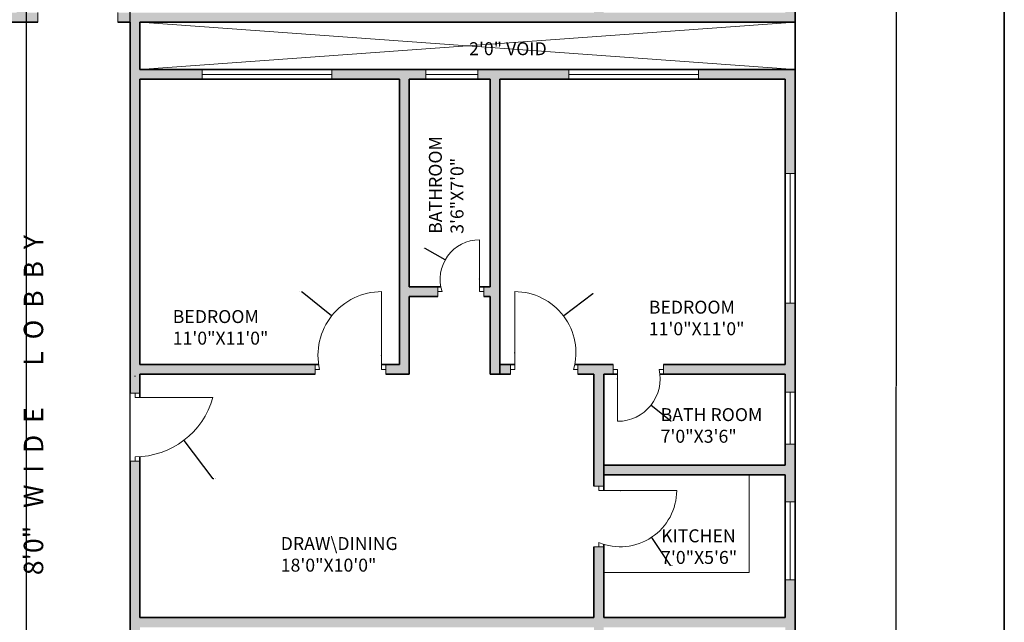
# Model space of a CAD drawing. Units: inches. Extents: x 2314 to 3223, y 1382 to 2735.
# Tile 11 of 14: x 2767 to 3223, y 1864 to 2143. Entities that reach past the tile are written whole.
import ezdxf

# ---------------------------------------------------------------- set-up
doc = ezdxf.new("R2010")
doc.units = ezdxf.units.IN
for name, color, linetype, lineweight in [('A-ANNO-DIMS', 2, 'Continuous', 18), ('A-ANNO-TTLB', 7, 'Continuous', 35), ('A-AREA-IDEN', 7, 'Continuous', 18), ('A-DOOR', 3, 'Continuous', 18), ('A-FLOR-FIXT', 8, 'Continuous', 18), ('A-FLOR-OPEN', 8, 'Continuous', 13), ('A-GLAZ', 4, 'Continuous', 18), ('A-WALL', 7, 'Continuous', 35)]:
    doc.layers.add(name, color=color, linetype=linetype, lineweight=lineweight)
doc.layers.add('A-WALL-PATT', color=251, linetype='Continuous', lineweight=13, true_color=0x636466)
doc.styles.get("Standard").update_dxf_attribs({"font": 'arial.ttf'})
doc.dimstyles.get("Standard").update_dxf_attribs({"dimtxt": 0.18, "dimasz": 0.18, "dimexe": 0.18, "dimexo": 0.0625, "dimgap": 0.09, "dimtad": 0, "dimtih": 1, "dimtoh": 1, "dimdec": 4, "dimzin": 0, "dimdsep": 46, "dimtxsty": 'Standard', "dimcen": 0.09, "dimadec": 0, "dimazin": 0, "dimtfac": 1, "dimtdec": 4, "dimtofl": 0, "dimtmove": 0, "dimatfit": 3, "dimfxl": 1, "dimtolj": 1, "dimtzin": 0, "dimarcsym": 0})

# ---------------------------------------------------------------- blocks, each defined once
blk = doc.blocks.new('WIN-PLAN-24')
for p, q in [((0, 24), (4.5, 24)), ((4.5, 24), (2.25, 24)), ((2.25, 24), (2.25, 0)), ((2.25, 0), (0, 0)), ((0, 0), (4.5, 0))]:
    blk.add_line(p, q)
blk = doc.blocks.new('WIN-PLAN-60')
for p, q in [((0, 4.5), (0, 0)), ((0, 0), (0, 2.25)), ((0, 2.25), (60, 2.25)), ((60, 2.25), (60, 4.5)), ((60, 4.5), (60, 0))]:
    blk.add_line(p, q)
blk = doc.blocks.new('WIN-PLAN-36')
for p, q in [((0, 36), (4.5, 36)), ((4.5, 36), (2.25, 36)), ((2.25, 36), (2.25, 0)), ((2.25, 0), (0, 0)), ((0, 0), (4.5, 0))]:
    blk.add_line(p, q)
blk = doc.blocks.new('*D30')
at = {"layer": 'A-ANNO-DIMS', "color": 0, "lineweight": -2, "transparency": 16777216}
for p, q in [((3125.96, 2381.78), (3172.77, 2381.78)), ((3172.59, 2381.6), (3172.59, 1973.38)), ((3172.59, 1564.8), (3172.59, 1973.02)), ((2822.96, 1564.62), (3172.77, 1564.62))]:
    blk.add_line(p, q, dxfattribs=at)
at = {"layer": 'A-ANNO-DIMS', "color": 0, "transparency": 16777216}
for points in [[(3172.56, 2381.6), (3172.62, 2381.6), (3172.59, 2381.78)], [(3172.56, 1564.8), (3172.62, 1564.8), (3172.59, 1564.62)]]:
    blk.add_solid(points, dxfattribs=at)
at = {"layer": 'Defpoints', "color": 0, "transparency": 16777216}
for p in [(3125.89, 2381.78), (2822.89, 1564.62), (3172.59, 1564.62)]:
    blk.add_point(p, dxfattribs=at)
at = {"layer": 'A-ANNO-DIMS', "color": 0, "transparency": 16777216, "insert": (3172.59, 1973.2), "char_height": 0.18, "attachment_point": 5}
blk.add_mtext('\\A1;817.2', dxfattribs=at)
blk = doc.blocks.new('*D39')
at = {"layer": 'A-ANNO-DIMS', "color": 0, "lineweight": -2, "transparency": 16777216}
for p, q in [((2770.39, 1744.06), (2770.39, 2428.66)), ((2770.57, 2428.48), (2794.17, 2428.48)), ((2818.21, 2428.48), (2794.62, 2428.48)), ((2818.39, 1744.06), (2818.39, 2428.66))]:
    blk.add_line(p, q, dxfattribs=at)
at = {"layer": 'A-ANNO-DIMS', "color": 0, "transparency": 16777216}
for points in [[(2770.57, 2428.51), (2770.57, 2428.45), (2770.39, 2428.48)], [(2818.21, 2428.51), (2818.21, 2428.45), (2818.39, 2428.48)]]:
    blk.add_solid(points, dxfattribs=at)
at = {"layer": 'Defpoints', "color": 0, "transparency": 16777216}
for p in [(2818.39, 2428.48), (2770.39, 1744), (2818.39, 1744)]:
    blk.add_point(p, dxfattribs=at)
at = {"layer": 'A-ANNO-DIMS', "color": 0, "transparency": 16777216, "insert": (2794.39, 2428.48), "char_height": 0.18, "attachment_point": 5}
blk.add_mtext('\\A1;48', dxfattribs=at)
blk = doc.blocks.new('*D61')
at = {"layer": 'A-ANNO-DIMS', "color": 0, "lineweight": -2, "transparency": 16777216}
for p, q in [((2820.55, 1978.07), (2820.73, 1978.07)), ((2820.64, 1977.98), (2820.64, 1978.16)), ((2856.84, 1930.53), (2843.38, 1948.21)), ((2857.02, 1930.53), (2856.84, 1930.53))]:
    blk.add_line(p, q, dxfattribs=at)
at = {"layer": 'A-ANNO-DIMS', "color": 0, "transparency": 16777216}
blk.add_solid([(2843.4, 1948.23), (2843.35, 1948.19), (2843.27, 1948.35)], dxfattribs=at)
at = {"layer": 'Defpoints', "color": 0, "transparency": 16777216}
for p in [(2820.64, 1978.07), (2843.27, 1948.35)]:
    blk.add_point(p, dxfattribs=at)
at = {"layer": 'A-ANNO-DIMS', "color": 0, "transparency": 16777216, "insert": (2857.57, 1930.53), "char_height": 0.18, "attachment_point": 5}
blk.add_mtext('\\A1;R37.346', dxfattribs=at)
blk = doc.blocks.new('*D69')
at = {"layer": 'A-ANNO-DIMS', "color": 0, "lineweight": -2, "transparency": 16777216}
for p, q in [((2897.68, 2017.07), (2897.86, 2017.07)), ((2897.86, 2017.07), (2911.54, 2006.16)), ((2934.61, 1987.68), (2934.79, 1987.68)), ((2934.7, 1987.59), (2934.7, 1987.77))]:
    blk.add_line(p, q, dxfattribs=at)
at = {"layer": 'A-ANNO-DIMS', "color": 0, "transparency": 16777216}
blk.add_solid([(2911.55, 2006.18), (2911.52, 2006.14), (2911.68, 2006.05)], dxfattribs=at)
at = {"layer": 'Defpoints', "color": 0, "transparency": 16777216}
for p in [(2911.68, 2006.05), (2934.7, 1987.68)]:
    blk.add_point(p, dxfattribs=at)
at = {"layer": 'A-ANNO-DIMS', "color": 0, "transparency": 16777216, "insert": (2897.13, 2017.07), "char_height": 0.18, "attachment_point": 5}
blk.add_mtext('\\A1;R29.454', dxfattribs=at)
blk = doc.blocks.new('*D73')
at = {"layer": 'A-ANNO-DIMS', "color": 0, "lineweight": -2, "transparency": 16777216}
for p, q in [((3032.35, 2016.16), (3018.95, 2006.02)), ((3032.53, 2016.16), (3032.35, 2016.16)), ((2996.14, 1988.83), (2996.32, 1988.83)), ((2996.23, 1988.74), (2996.23, 1988.92))]:
    blk.add_line(p, q, dxfattribs=at)
at = {"layer": 'A-ANNO-DIMS', "color": 0, "transparency": 16777216}
blk.add_solid([(3018.93, 2006.04), (3018.97, 2005.99), (3018.81, 2005.91)], dxfattribs=at)
at = {"layer": 'Defpoints', "color": 0, "transparency": 16777216}
for p in [(3018.81, 2005.91), (2996.23, 1988.83)]:
    blk.add_point(p, dxfattribs=at)
at = {"layer": 'A-ANNO-DIMS', "color": 0, "transparency": 16777216, "insert": (3032.99, 2016.16), "char_height": 0.18, "attachment_point": 5}
blk.add_mtext('\\A1;R28.31', dxfattribs=at)
blk = doc.blocks.new('*D79')
at = {"layer": 'A-ANNO-DIMS', "color": 0, "lineweight": -2, "transparency": 16777216}
for p, q in [((3045.03, 1925.13), (3045.21, 1925.13)), ((3045.12, 1925.04), (3045.12, 1925.22)), ((3068.24, 1890.5), (3059.67, 1903.33)), ((3068.42, 1890.5), (3068.24, 1890.5))]:
    blk.add_line(p, q, dxfattribs=at)
at = {"layer": 'A-ANNO-DIMS', "color": 0, "transparency": 16777216}
blk.add_solid([(3059.69, 1903.35), (3059.64, 1903.32), (3059.57, 1903.48)], dxfattribs=at)
at = {"layer": 'Defpoints', "color": 0, "transparency": 16777216}
for p in [(3045.12, 1925.13), (3059.57, 1903.48)]:
    blk.add_point(p, dxfattribs=at)
at = {"layer": 'A-ANNO-DIMS', "color": 0, "transparency": 16777216, "insert": (3068.9, 1890.5), "char_height": 0.18, "attachment_point": 5}
blk.add_mtext('\\A1;R26.02', dxfattribs=at)
blk = doc.blocks.new('*D88')
at = {"layer": 'A-ANNO-DIMS', "color": 0, "lineweight": -2, "transparency": 16777216}
for p, q in [((3043.74, 1976.79), (3043.92, 1976.79)), ((3043.83, 1976.7), (3043.83, 1976.88)), ((3068.4, 1957.16), (3059.33, 1964.41)), ((3068.58, 1957.16), (3068.4, 1957.16))]:
    blk.add_line(p, q, dxfattribs=at)
at = {"layer": 'A-ANNO-DIMS', "color": 0, "transparency": 16777216}
blk.add_solid([(3059.35, 1964.43), (3059.31, 1964.39), (3059.19, 1964.52)], dxfattribs=at)
at = {"layer": 'Defpoints', "color": 0, "transparency": 16777216}
for p in [(3043.83, 1976.79), (3059.19, 1964.52)]:
    blk.add_point(p, dxfattribs=at)
at = {"layer": 'A-ANNO-DIMS', "color": 0, "transparency": 16777216, "insert": (3069.13, 1957.16), "char_height": 0.18, "attachment_point": 5}
blk.add_mtext('\\A1;R19.658', dxfattribs=at)
blk = doc.blocks.new('*D93')
at = {"layer": 'A-ANNO-DIMS', "color": 0, "lineweight": -2, "transparency": 16777216}
for p, q in [((2954.46, 2037.31), (2954.64, 2037.31)), ((2954.64, 2037.31), (2963.96, 2032.02)), ((2979.83, 2022.97), (2980.01, 2022.97)), ((2979.92, 2022.88), (2979.92, 2023.06))]:
    blk.add_line(p, q, dxfattribs=at)
at = {"layer": 'A-ANNO-DIMS', "color": 0, "transparency": 16777216}
blk.add_solid([(2963.98, 2032.05), (2963.95, 2031.99), (2964.12, 2031.93)], dxfattribs=at)
at = {"layer": 'Defpoints', "color": 0, "transparency": 16777216}
for p in [(2964.12, 2031.93), (2979.92, 2022.97)]:
    blk.add_point(p, dxfattribs=at)
at = {"layer": 'A-ANNO-DIMS', "color": 0, "transparency": 16777216, "insert": (2953.91, 2037.31), "char_height": 0.18, "attachment_point": 5}
blk.add_mtext('\\A1;R18.168', dxfattribs=at)

msp = doc.modelspace()

# ---------------------------------------------------------------- hatches: boundary and pattern name
at = {"layer": 'A-WALL-PATT'}
h = msp.add_hatch(color=256, dxfattribs=at)
h.dxf.hatch_style = 1
h.paths.add_polyline_path([(2443.3302, 2379.5332), (2443.3302, 2381.7832), (2410.3927, 2381.7832), (2410.3927, 2336.7008), (2414.8927, 2336.7008), (2414.8927, 2377.2832), (2443.3302, 2377.2832)])
h.paths.add_polyline_path([(2561.3645, 2379.5332), (2561.3645, 2381.7832), (2503.3302, 2381.7832), (2503.3302, 2377.2832), (2546.8927, 2377.2832), (2546.8927, 2245.2832), (2541.8787, 2245.2832), (2541.8787, 2240.7832), (2551.3927, 2240.7832), (2551.3927, 2377.2832), (2561.3645, 2377.2832)])
h.paths.add_polyline_path([(2656.0607, 2381.7832), (2597.3645, 2381.7832), (2597.3645, 2377.2832), (2617.3927, 2377.2832), (2617.3927, 2257.2832), (2584.2532, 2257.2832), (2584.2532, 2252.7832), (2625.8528, 2252.7832), (2625.8528, 2255.0332), (2625.8528, 2257.2832), (2621.8927, 2257.2832), (2621.8927, 2377.2832), (2656.0607, 2377.2832), (2656.0607, 2379.5332)])
h.paths.add_polyline_path([(2807.3418, 2381.7832), (2716.0607, 2381.7832), (2716.0607, 2377.2832), (2765.8927, 2377.2832), (2765.8927, 2257.2832), (2661.6935, 2257.2832), (2661.6935, 2252.7832), (2765.8927, 2252.7832), (2765.8927, 2146.2832), (2760.9259, 2146.2832), (2760.9259, 2141.8832), (2775.7119, 2141.8832), (2775.7119, 2146.2832), (2770.3927, 2146.2832), (2770.3927, 2252.7832), (2877.684, 2252.7832), (2877.684, 2255.0332), (2877.684, 2257.2832), (2770.3927, 2257.2832), (2770.3927, 2377.2832), (2807.3418, 2377.2832), (2807.3418, 2379.5332)])
h.paths.add_polyline_path([(2937.2118, 2381.7832), (2867.3418, 2381.7832), (2867.3418, 2377.2832), (2914.3927, 2377.2832), (2914.3927, 2257.2832), (2908.4124, 2257.2832), (2908.4124, 2252.7832), (2960.6432, 2252.7832), (2960.6432, 2255.0332), (2960.6432, 2257.2832), (2918.8927, 2257.2832), (2918.8927, 2377.2832), (2937.2118, 2377.2832)])
h.paths.add_polyline_path([(3022.1601, 2381.7832), (2973.2118, 2381.7832), (2973.2118, 2379.5332), (2973.2118, 2377.2832), (2984.8927, 2377.2832), (2984.8927, 2257.2832), (2980.0601, 2257.2832), (2980.0601, 2252.7832), (2984.8927, 2252.7832), (2984.8927, 2240.7832), (2995.668, 2240.7832), (2995.668, 2243.0332), (2995.668, 2245.2832), (2989.3927, 2245.2832), (2989.3927, 2377.2832), (3022.1601, 2377.2832), (3022.1601, 2379.5332)])
h.paths.add_polyline_path([(3125.8927, 2381.7832), (3082.1601, 2381.7832), (3082.1601, 2377.2832), (3121.3927, 2377.2832), (3121.3927, 2334.7388), (3125.8927, 2334.7388)])
h.paths.add_polyline_path([(3125.8927, 2274.7388), (3121.3927, 2274.7388), (3121.3927, 2245.2832), (3066.4832, 2245.2832), (3066.4832, 2240.7832), (3121.3927, 2240.7832), (3121.3927, 2232.1868), (3125.8927, 2232.1868)])
h.paths.add_polyline_path([(3125.8927, 2208.1868), (3121.3927, 2208.1868), (3121.3927, 2198.7832), (3037.3927, 2198.7832), (3037.3927, 2240.7832), (3041.2694, 2240.7832), (3041.2694, 2243.0332), (3041.2694, 2245.2832), (3026.8205, 2245.2832), (3026.8205, 2240.7832), (3032.8927, 2240.7832), (3032.8927, 2190.4022), (3037.3927, 2190.4022), (3037.3927, 2194.2832), (3121.3927, 2194.2832), (3121.3927, 2182.1835), (3125.8927, 2182.1835)])
h.paths.add_polyline_path([(3125.8927, 2158.1835), (3121.3927, 2158.1835), (3121.3927, 2146.2832), (3037.3927, 2146.2832), (3037.3927, 2169.3726), (3035.1427, 2169.3726), (3032.8927, 2169.3726), (3032.8927, 2146.2832), (2812.7301, 2146.2832), (2812.7301, 2144.0832), (2812.7301, 2141.8832), (2818.3927, 2141.8832), (2818.3927, 1970.1316), (2822.8927, 1970.1316), (2822.8927, 1978.8832), (2903.9846, 1978.8832), (2903.9846, 1981.1332), (2903.9846, 1983.3832), (2822.8927, 1983.3832), (2822.8927, 2115.3832), (2851.7162, 2115.3832), (2851.7162, 2117.6332), (2851.7162, 2119.8832), (2822.8927, 2119.8832), (2822.8927, 2141.8832), (3125.8927, 2141.8832)])
h.paths.add_polyline_path([(3125.8927, 2119.8832), (3081.193, 2119.8832), (3081.193, 2115.3832), (3121.3927, 2115.3832), (3121.3927, 2071.8188), (3125.8927, 2071.8188)], flags=17)
h.paths.add_polyline_path([(2989.3927, 2115.3832), (3021.193, 2115.3832), (3021.193, 2117.6332), (3021.193, 2119.8832), (2979.123, 2119.8832), (2979.123, 2115.3832), (2984.8927, 2115.3832), (2984.8927, 2019.3832), (2981.9225, 2019.3832), (2981.9225, 2014.8832), (2984.8927, 2014.8832), (2984.8927, 1983.3832), (2984.8927, 1978.8832), (2989.3927, 1978.8832), (2989.3927, 1983.3832)], flags=17)
h.paths.add_polyline_path([(2947.3927, 2115.3832), (2955.123, 2115.3832), (2955.123, 2117.6332), (2955.123, 2119.8832), (2911.7162, 2119.8832), (2911.7162, 2115.3832), (2942.8927, 2115.3832), (2942.8927, 1983.3832), (2936.7017, 1983.3832), (2936.7017, 1978.8832), (2947.3927, 1978.8832), (2947.3927, 1983.3832), (2947.3927, 2014.8832), (2960.7167, 2014.8832), (2960.7167, 2017.1332), (2960.7167, 2019.3832), (2947.3927, 2019.3832)], flags=17)
h.paths.add_polyline_path([(3037.3927, 1978.8832), (3041.8276, 1978.8832), (3041.8276, 1981.1332), (3041.8276, 1983.3832), (3025.477, 1983.3832), (3025.477, 1978.8832), (3032.8927, 1978.8832), (3032.8927, 1927.1259), (3035.1427, 1927.1259), (3037.3927, 1927.1259)])
h.paths.add_polyline_path([(3125.8927, 2011.8188), (3123.6427, 2011.8188), (3121.3927, 2011.8188), (3121.3927, 1983.3832), (3065, 1983.3832), (3065, 1978.8832), (3121.3927, 1978.8832), (3121.3927, 1970.5932), (3125.8927, 1970.5932)], flags=17)
h.paths.add_polyline_path([(2994.2341, 1983.3832), (2989.3927, 1983.3832), (2989.3927, 1978.8832), (2994.2341, 1978.8832), (2994.2341, 1981.1332)], flags=16)
h.paths.add_polyline_path([(3125.8927, 1946.5932), (3121.3927, 1946.5932), (3121.3927, 1936.8832), (3037.3927, 1936.8832), (3037.3927, 1932.3832), (3121.3927, 1932.3832), (3121.3927, 1919.825), (3125.8927, 1919.825)])
h.paths.add_polyline_path([(3125.8927, 1883.825), (3121.3927, 1883.825), (3121.3927, 1866.3832), (3037.3927, 1866.3832), (3037.3927, 1899.0954), (3035.1427, 1899.0954), (3032.8927, 1899.0954), (3032.8927, 1866.3832), (2822.8927, 1866.3832), (2822.8927, 1938.7212), (2820.6427, 1938.7212), (2818.3927, 1938.7212), (2818.3927, 1786.9239), (2822.8927, 1786.9239), (2822.8927, 1861.8832), (3032.8927, 1861.8832), (3032.8927, 1825.1023), (3037.3927, 1825.1023), (3037.3927, 1861.8832), (3121.3927, 1861.8832), (3121.3927, 1844.6765), (3125.8927, 1844.6765)])
h.paths.add_polyline_path([(3125.8927, 1808.6765), (3121.3927, 1808.6765), (3121.3927, 1795.8832), (3037.3927, 1795.8832), (3037.3927, 1799.4755), (3032.8927, 1799.4755), (3032.8927, 1749.3832), (3026.5034, 1749.3832), (3026.5034, 1744.8832), (3032.8927, 1744.8832), (3034.9255, 1744.8832), (3043.1326, 1744.8832), (3043.1326, 1747.1332), (3043.1326, 1749.3832), (3037.3927, 1749.3832), (3037.3927, 1791.3832), (3121.3927, 1791.3832), (3121.3927, 1783.3103), (3125.8927, 1783.3103)])
h.paths.add_polyline_path([(3125.8927, 1759.3103), (3121.3927, 1759.3103), (3121.3927, 1749.3832), (3065.1845, 1749.3832), (3065.1845, 1744.8832), (3121.3927, 1744.8832), (3121.3927, 1709.3573), (3125.8927, 1709.3573)])
h.paths.add_polyline_path([(3125.8927, 1649.3573), (3121.3927, 1649.3573), (3121.3927, 1612.8832), (3095.116, 1612.8832), (3095.116, 1608.3832), (3125.8927, 1608.3832)])
h.paths.add_polyline_path([(3035.116, 1612.8832), (2993.8927, 1612.8832), (2993.8927, 1744.8832), (2998.7409, 1744.8832), (2998.7409, 1749.3832), (2989.3927, 1749.3832), (2989.3927, 1744.8832), (2989.3927, 1701.3832), (2972.8226, 1701.3832), (2972.8226, 1696.8832), (2989.3927, 1696.8832), (2989.3927, 1612.8832), (2978.2225, 1612.8832), (2978.2225, 1608.3832), (3035.116, 1608.3832), (3035.116, 1610.6332)])
h.paths.add_polyline_path([(2947.3927, 1696.8832), (2950.7566, 1696.8832), (2950.7566, 1699.1332), (2950.7566, 1701.3832), (2947.3927, 1701.3832), (2947.3927, 1744.8832), (2947.3927, 1749.3832), (2937.649, 1749.3832), (2937.649, 1744.8832), (2942.8927, 1744.8832), (2942.8927, 1612.8832), (2907.783, 1612.8832), (2907.783, 1608.3832), (2954.2225, 1608.3832), (2954.2225, 1610.6332), (2954.2225, 1612.8832), (2947.3927, 1612.8832)])
h.paths.add_polyline_path([(2822.8927, 1744.8832), (2905.3491, 1744.8832), (2905.3491, 1747.1332), (2905.3491, 1749.3832), (2822.8927, 1749.3832), (2822.8927, 1756.9185), (2818.3927, 1756.9185), (2818.3927, 1612.8832), (2818.3927, 1569.1205), (2722.3927, 1569.1205), (2722.3927, 1612.8832), (2722.3927, 1756.9185), (2717.8927, 1756.9185), (2717.8927, 1750.0143), (2633.6297, 1750.0143), (2633.6437, 1745.2665), (2717.8927, 1745.5143), (2717.8927, 1612.8832), (2689.8467, 1612.8832), (2689.8467, 1608.3832), (2717.8927, 1608.3832), (2717.8927, 1564.6205), (2722.3927, 1564.6205), (2822.8927, 1564.6205), (2822.8927, 1569.1205), (2822.8927, 1608.3832), (2847.783, 1608.3832), (2847.783, 1610.6332), (2847.783, 1612.8832), (2822.8927, 1612.8832)])
h.paths.add_polyline_path([(2629.8467, 1612.8832), (2597.8927, 1612.8832), (2597.8927, 1744.8832), (2597.8927, 1745.1613), (2601.5887, 1745.1721), (2601.5816, 1747.5932), (2601.5745, 1750.0143), (2593.3927, 1750.0143), (2593.3927, 1744.8832), (2593.3927, 1713.3832), (2589.7588, 1713.3832), (2589.7588, 1708.8832), (2593.3927, 1708.8832), (2593.3927, 1612.8832), (2582.3793, 1612.8832), (2582.3793, 1608.3832), (2629.8467, 1608.3832), (2629.8467, 1610.6332)])
h.paths.add_polyline_path([(2551.3927, 1708.8832), (2567.6776, 1708.8832), (2567.6776, 1711.1332), (2567.6776, 1713.3832), (2551.3927, 1713.3832), (2551.3927, 1744.8832), (2551.3927, 1750.0143), (2543.5657, 1750.0143), (2543.5657, 1747.5079), (2543.5657, 1745.0014), (2546.8927, 1745.0112), (2546.8927, 1744.8832), (2546.8927, 1612.8832), (2502.9339, 1612.8832), (2502.9339, 1608.3832), (2558.3793, 1608.3832), (2558.3793, 1610.6332), (2558.3793, 1612.8832), (2551.3927, 1612.8832)])
h.paths.add_polyline_path([(2414.8927, 1656.2547), (2410.3927, 1656.2547), (2410.3927, 1608.3832), (2442.9339, 1608.3832), (2442.9339, 1610.6332), (2442.9339, 1612.8832), (2414.8927, 1612.8832)])
h.paths.add_polyline_path([(2414.8927, 1744.8832), (2468.8906, 1744.8832), (2468.8906, 1747.1332), (2468.8906, 1749.3832), (2414.8927, 1749.3832), (2414.8927, 1757.7622), (2410.3927, 1757.7622), (2410.3927, 1716.2547), (2414.8927, 1716.2547)])
h.paths.add_polyline_path([(2414.8927, 1791.3832), (2498.8927, 1791.3832), (2498.8927, 1749.3832), (2492.9799, 1749.3832), (2492.9799, 1744.8832), (2498.8927, 1744.8832), (2503.3927, 1744.8832), (2508.0135, 1744.8968), (2508.0059, 1747.4556), (2507.9984, 1750.0143), (2503.3927, 1750.0143), (2503.3927, 1802.6362), (2501.1427, 1802.6362), (2498.8927, 1802.6362), (2498.8927, 1795.8832), (2414.8927, 1795.8832), (2414.8927, 1808.0943), (2410.3927, 1808.0943), (2410.3927, 1781.7622), (2414.8927, 1781.7622)])
h.paths.add_polyline_path([(2722.3927, 1937.589), (2720.1427, 1937.589), (2717.8927, 1937.589), (2717.8927, 1866.3832), (2503.3927, 1866.3832), (2503.3927, 1896.3484), (2498.8927, 1896.3484), (2498.8927, 1866.3832), (2414.8927, 1866.3832), (2414.8927, 1882.1496), (2410.3927, 1882.1496), (2410.3927, 1844.0943), (2414.8927, 1844.0943), (2414.8927, 1861.8832), (2498.8927, 1861.8832), (2498.8927, 1831.4783), (2501.1427, 1831.4783), (2503.3927, 1831.4783), (2503.3927, 1861.8832), (2717.8927, 1861.8832), (2717.8927, 1786.9239), (2722.3927, 1786.9239)])
h.paths.add_polyline_path([(2414.8927, 1932.3832), (2498.8927, 1932.3832), (2498.8927, 1924.7883), (2503.3927, 1924.7883), (2503.3927, 1978.8832), (2505.8599, 1978.8832), (2505.8599, 1981.1332), (2505.8599, 1983.3832), (2493.3697, 1983.3832), (2493.3697, 1978.8832), (2498.8927, 1978.8832), (2498.8927, 1936.8832), (2414.8927, 1936.8832), (2414.8927, 1943.2834), (2410.3927, 1943.2834), (2410.3927, 1918.1496), (2414.8927, 1918.1496)])
h.paths.add_polyline_path([(2414.8927, 2020.3133), (2412.6427, 2020.3133), (2410.3927, 2020.3133), (2410.3927, 1967.2834), (2414.8927, 1967.2834), (2414.8927, 1978.8832), (2468.8513, 1978.8832), (2468.8513, 1981.1332), (2468.8513, 1983.3832), (2414.8927, 1983.3832)])
h.paths.add_polyline_path([(2414.8927, 2115.3832), (2453.004, 2115.3832), (2453.004, 2117.6332), (2453.004, 2119.8832), (2410.3927, 2119.8832), (2410.3927, 2080.3133), (2414.8927, 2080.3133)], flags=17)
h.paths.add_polyline_path([(2559.0969, 2117.6332), (2559.0969, 2119.8832), (2513.004, 2119.8832), (2513.004, 2115.3832), (2546.8927, 2115.3832), (2546.8927, 1983.3832), (2542.7531, 1983.3832), (2542.7531, 1978.8832), (2551.3927, 1978.8832), (2551.3927, 2014.8832), (2570.3098, 2014.8832), (2570.3098, 2017.1332), (2570.3098, 2019.3832), (2551.3927, 2019.3832), (2551.3927, 2115.3832), (2559.0969, 2115.3832)], flags=17)
h.paths.add_polyline_path([(2628.5073, 2117.6332), (2628.5073, 2119.8832), (2583.0969, 2119.8832), (2583.0969, 2115.3832), (2593.3927, 2115.3832), (2593.3927, 2019.3832), (2590.2108, 2019.3832), (2590.2108, 2014.8832), (2593.3927, 2014.8832), (2593.3927, 1978.8832), (2601.5907, 1978.8832), (2601.5907, 1981.1332), (2601.5907, 1983.3832), (2597.8927, 1983.3832), (2597.8927, 2115.3832), (2628.5073, 2115.3832)], flags=17)
h.paths.add_polyline_path([(2722.3927, 2141.8832), (2726.9871, 2141.8832), (2726.9871, 2144.2705), (2726.9871, 2146.2832), (2503.3927, 2146.2832), (2503.3927, 2168.2161), (2501.1427, 2168.2161), (2498.8927, 2168.2161), (2498.8927, 2146.2832), (2414.8927, 2146.2832), (2414.8927, 2156.5041), (2410.3927, 2156.5041), (2410.3927, 2141.8832), (2717.8927, 2141.8832), (2717.8927, 2119.8832), (2688.5073, 2119.8832), (2688.5073, 2115.3832), (2717.8927, 2115.3832), (2717.8927, 1983.3832), (2633.2454, 1983.3832), (2633.2454, 1978.8832), (2717.8927, 1978.8832), (2717.8927, 1970.1316), (2720.1427, 1970.1316), (2722.3927, 1970.1316)])
h.paths.add_polyline_path([(2557.3704, 1462.9278), (2940.0934, 1462.9278), (2940.0934, 1512.3848), (2557.3704, 1512.3848)], flags=9)
h.paths.add_polyline_path([(2846.2527, 1703.1384), (2892.8612, 1703.1384), (2892.8612, 1725.5272), (2846.2527, 1725.5272)], flags=25)
h.paths.add_polyline_path([(2885.6102, 1812.1147), (2946.1505, 1812.1147), (2946.1505, 1834.5035), (2885.6102, 1834.5035)], flags=25)
h.paths.add_polyline_path([(2885.6102, 1884.183), (2946.1505, 1884.183), (2946.1505, 1906.5718), (2885.6102, 1906.5718)], flags=25)
h.paths.add_polyline_path([(3066.365, 1705.5431), (3112.9735, 1705.5431), (3112.9735, 1727.9319), (3066.365, 1727.9319)], flags=9)
h.paths.add_polyline_path([(3061.8255, 1887.7513), (3101.6154, 1887.7513), (3101.6154, 1910.1401), (3061.8255, 1910.1401)], flags=25)
h.paths.add_polyline_path([(3063.3679, 1816.2121), (3103.1578, 1816.2121), (3103.1578, 1838.6009), (3063.3679, 1838.6009)], flags=25)
h.paths.add_polyline_path([(3053.3743, 1768.416), (3107.1329, 1768.416), (3107.1329, 1790.8048), (3053.3743, 1790.8048)], flags=25)
h.paths.add_polyline_path([(3061.6068, 1943.822), (3115.3653, 1943.822), (3115.3653, 1966.2109), (3061.6068, 1966.2109)], flags=9)
h.paths.add_polyline_path([(2745.0978, 1763.6604), (2797.9354, 1763.6604), (2797.9354, 1776.0247), (2745.0978, 1776.0247)], flags=9)
h.paths.add_polyline_path([(2574.2135, 1819.2586), (2634.7538, 1819.2586), (2634.7538, 1841.6474), (2574.2135, 1841.6474)], flags=25)
h.paths.add_polyline_path([(2574.2135, 1891.3269), (2634.7538, 1891.3269), (2634.7538, 1913.7157), (2574.2135, 1913.7157)], flags=25)
h.paths.add_polyline_path([(2638.4466, 1702.43), (2685.0551, 1702.43), (2685.0551, 1724.8188), (2638.4466, 1724.8188)], flags=25)
h.paths.add_polyline_path([(2435.9715, 1697.1215), (2482.5799, 1697.1215), (2482.5799, 1719.5103), (2435.9715, 1719.5103)], flags=9)
h.paths.add_polyline_path([(2431.2046, 1893.7833), (2470.9945, 1893.7833), (2470.9945, 1916.1721), (2431.2046, 1916.1721)], flags=25)
h.paths.add_polyline_path([(2439.8144, 1817.2116), (2479.6043, 1817.2116), (2479.6043, 1839.6004), (2439.8144, 1839.6004)], flags=25)
h.paths.add_polyline_path([(2441.2607, 1753.0942), (2495.0192, 1753.0942), (2495.0192, 1775.483), (2441.2607, 1775.483)], flags=25)
h.paths.add_polyline_path([(2421.216, 1945.3109), (2474.9746, 1945.3109), (2474.9746, 1967.6997), (2421.216, 1967.6997)], flags=25)
h.paths.add_polyline_path([(2585.4464, 1627.5703), (2585.4464, 1679), (2563.0576, 1679), (2563.0576, 1627.5703)], flags=9)
h.paths.add_polyline_path([(2978.3497, 1618.7039), (2978.3497, 1670.1337), (2955.9609, 1670.1337), (2955.9609, 1618.7039)], flags=9)
h.paths.add_polyline_path([(2975.9502, 2041.7828), (2975.9502, 2093.2125), (2953.5614, 2093.2125), (2953.5614, 2041.7828)], flags=25)
h.paths.add_polyline_path([(2835.6537, 1989.2068), (2882.2621, 1989.2068), (2882.2621, 2011.5956), (2835.6537, 2011.5956)], flags=25)
h.paths.add_polyline_path([(2649.3769, 1997.5659), (2695.9853, 1997.5659), (2695.9853, 2019.9547), (2649.3769, 2019.9547)], flags=25)
h.paths.add_polyline_path([(2579.9087, 2040.3429), (2579.9087, 2091.7726), (2557.5198, 2091.7726), (2557.5198, 2040.3429)], flags=25)
h.paths.add_polyline_path([(2783.2404, 1883.1956), (2783.2404, 2067.1369), (2764.694, 2067.1369), (2764.694, 1883.1956)], flags=9)
h.paths.add_polyline_path([(3055.8435, 1993.5571), (3102.4519, 1993.5571), (3102.4519, 2015.9459), (3055.8435, 2015.9459)], flags=25)
h.paths.add_polyline_path([(2423.6009, 1984.6082), (2470.2094, 1984.6082), (2470.2094, 2006.997), (2423.6009, 2006.997)], flags=25)
h.paths.add_polyline_path([(2973.4115, 2123.1668), (3013.1319, 2123.1668), (3013.1319, 2135.531), (2973.4115, 2135.531)], flags=25)
h.paths.add_polyline_path([(2534.3846, 2124.6231), (2574.105, 2124.6231), (2574.105, 2136.9874), (2534.3846, 2136.9874)], flags=25)
h.paths.add_polyline_path([(2829.1368, 2188.1931), (2889.411, 2188.1931), (2889.411, 2210.5819), (2829.1368, 2210.5819)], flags=9)
h.paths.add_polyline_path([(2633.2547, 2185.0437), (2693.5289, 2185.0437), (2693.5289, 2207.4325), (2633.2547, 2207.4325)], flags=9)
h.paths.add_polyline_path([(2445.1812, 2167.0395), (2496.611, 2167.0395), (2496.611, 2189.4284), (2445.1812, 2189.4284)], flags=9)
h.paths.add_polyline_path([(2429.1678, 2194.5482), (2480.5975, 2194.5482), (2480.5975, 2216.937), (2429.1678, 2216.937)], flags=9)
h.paths.add_polyline_path([(3060.1138, 2158.1056), (3111.5436, 2158.1056), (3111.5436, 2180.4944), (3060.1138, 2180.4944)], flags=9)
h.paths.add_polyline_path([(3055.6824, 2201.2631), (3107.1122, 2201.2631), (3107.1122, 2223.652), (3055.6824, 2223.652)], flags=25)
h.paths.add_polyline_path([(3044.3482, 2257.7345), (3090.9567, 2257.7345), (3090.9567, 2280.1233), (3044.3482, 2280.1233)], flags=9)
h.paths.add_polyline_path([(2942.5437, 2306.9625), (2982.3336, 2306.9625), (2982.3336, 2329.3513), (2942.5437, 2329.3513)], flags=9)
h.paths.add_polyline_path([(2799.5865, 2259.1663), (2846.195, 2259.1663), (2846.195, 2281.5551), (2799.5865, 2281.5551)], flags=25)
h.paths.add_polyline_path([(2670.4998, 2261.1493), (2717.1082, 2261.1493), (2717.1082, 2283.5381), (2670.4998, 2283.5381)], flags=25)
h.paths.add_polyline_path([(2553.0333, 2302.7735), (2592.8232, 2302.7735), (2592.8232, 2325.1624), (2553.0333, 2325.1624)], flags=9)
h.paths.add_polyline_path([(2432.0288, 2268.6489), (2478.6372, 2268.6489), (2478.6372, 2291.0377), (2432.0288, 2291.0377)], flags=9)
h = msp.add_hatch(color=256, dxfattribs=at)
h.dxf.hatch_style = 1
h.paths.add_polyline_path([(2503.3927, 2240.7832), (2507.7952, 2240.7832), (2507.7952, 2245.2832), (2496.4262, 2245.2832), (2496.4262, 2243.0332), (2496.4262, 2240.7832), (2498.8927, 2240.7832), (2498.8927, 2198.7832), (2414.8927, 2198.7832), (2414.8927, 2206.5718), (2410.3927, 2206.5718), (2410.3927, 2180.5041), (2412.6427, 2180.5041), (2414.8927, 2180.5041), (2414.8927, 2194.2832), (2498.8927, 2194.2832), (2498.8927, 2191.0069), (2503.3927, 2191.0069)])
h.paths.add_polyline_path([(2414.8927, 2276.7008), (2410.3927, 2276.7008), (2410.3927, 2230.5718), (2414.8927, 2230.5718), (2414.8927, 2240.7832), (2474.2564, 2240.7832), (2474.2564, 2243.0332), (2474.2564, 2245.2832), (2414.8927, 2245.2832)])
h.paths.add_polyline_path([(2557.3704, 1462.9278), (2940.0934, 1462.9278), (2940.0934, 1512.3848), (2557.3704, 1512.3848)], flags=9)
h.paths.add_polyline_path([(2846.2527, 1703.1384), (2892.8612, 1703.1384), (2892.8612, 1725.5272), (2846.2527, 1725.5272)], flags=9)
h.paths.add_polyline_path([(2885.6102, 1812.1147), (2946.1505, 1812.1147), (2946.1505, 1834.5035), (2885.6102, 1834.5035)], flags=9)
h.paths.add_polyline_path([(2885.6102, 1884.183), (2946.1505, 1884.183), (2946.1505, 1906.5718), (2885.6102, 1906.5718)], flags=9)
h.paths.add_polyline_path([(3066.365, 1705.5431), (3112.9735, 1705.5431), (3112.9735, 1727.9319), (3066.365, 1727.9319)], flags=9)
h.paths.add_polyline_path([(3061.8255, 1887.7513), (3101.6154, 1887.7513), (3101.6154, 1910.1401), (3061.8255, 1910.1401)], flags=9)
h.paths.add_polyline_path([(3063.3679, 1816.2121), (3103.1578, 1816.2121), (3103.1578, 1838.6009), (3063.3679, 1838.6009)], flags=9)
h.paths.add_polyline_path([(3053.3743, 1768.416), (3107.1329, 1768.416), (3107.1329, 1790.8048), (3053.3743, 1790.8048)], flags=9)
h.paths.add_polyline_path([(3061.6068, 1943.822), (3115.3653, 1943.822), (3115.3653, 1966.2109), (3061.6068, 1966.2109)], flags=9)
h.paths.add_polyline_path([(2745.0978, 1763.6604), (2797.9354, 1763.6604), (2797.9354, 1776.0247), (2745.0978, 1776.0247)], flags=9)
h.paths.add_polyline_path([(2574.2135, 1819.2586), (2634.7538, 1819.2586), (2634.7538, 1841.6474), (2574.2135, 1841.6474)], flags=9)
h.paths.add_polyline_path([(2574.2135, 1891.3269), (2634.7538, 1891.3269), (2634.7538, 1913.7157), (2574.2135, 1913.7157)], flags=9)
h.paths.add_polyline_path([(2638.4466, 1702.43), (2685.0551, 1702.43), (2685.0551, 1724.8188), (2638.4466, 1724.8188)], flags=9)
h.paths.add_polyline_path([(2435.9715, 1697.1215), (2482.5799, 1697.1215), (2482.5799, 1719.5103), (2435.9715, 1719.5103)], flags=9)
h.paths.add_polyline_path([(2431.2046, 1893.7833), (2470.9945, 1893.7833), (2470.9945, 1916.1721), (2431.2046, 1916.1721)], flags=9)
h.paths.add_polyline_path([(2439.8144, 1817.2116), (2479.6043, 1817.2116), (2479.6043, 1839.6004), (2439.8144, 1839.6004)], flags=9)
h.paths.add_polyline_path([(2441.2607, 1753.0942), (2495.0192, 1753.0942), (2495.0192, 1775.483), (2441.2607, 1775.483)], flags=9)
h.paths.add_polyline_path([(2421.216, 1945.3109), (2474.9746, 1945.3109), (2474.9746, 1967.6997), (2421.216, 1967.6997)], flags=9)
h.paths.add_polyline_path([(2585.4464, 1627.5703), (2585.4464, 1679), (2563.0576, 1679), (2563.0576, 1627.5703)], flags=9)
h.paths.add_polyline_path([(2978.3497, 1618.7039), (2978.3497, 1670.1337), (2955.9609, 1670.1337), (2955.9609, 1618.7039)], flags=9)
h.paths.add_polyline_path([(2975.9502, 2041.7828), (2975.9502, 2093.2125), (2953.5614, 2093.2125), (2953.5614, 2041.7828)], flags=9)
h.paths.add_polyline_path([(2835.6537, 1989.2068), (2882.2621, 1989.2068), (2882.2621, 2011.5956), (2835.6537, 2011.5956)], flags=9)
h.paths.add_polyline_path([(2649.3769, 1997.5659), (2695.9853, 1997.5659), (2695.9853, 2019.9547), (2649.3769, 2019.9547)], flags=9)
h.paths.add_polyline_path([(2579.9087, 2040.3429), (2579.9087, 2091.7726), (2557.5198, 2091.7726), (2557.5198, 2040.3429)], flags=9)
h.paths.add_polyline_path([(2783.2404, 1883.1956), (2783.2404, 2067.1369), (2764.694, 2067.1369), (2764.694, 1883.1956)], flags=9)
h.paths.add_polyline_path([(3055.8435, 1993.5571), (3102.4519, 1993.5571), (3102.4519, 2015.9459), (3055.8435, 2015.9459)], flags=9)
h.paths.add_polyline_path([(2423.6009, 1984.6082), (2470.2094, 1984.6082), (2470.2094, 2006.997), (2423.6009, 2006.997)], flags=9)
h.paths.add_polyline_path([(2973.4115, 2123.1668), (3013.1319, 2123.1668), (3013.1319, 2135.531), (2973.4115, 2135.531)], flags=9)
h.paths.add_polyline_path([(2534.3846, 2124.6231), (2574.105, 2124.6231), (2574.105, 2136.9874), (2534.3846, 2136.9874)], flags=9)
h.paths.add_polyline_path([(2829.1368, 2188.1931), (2889.411, 2188.1931), (2889.411, 2210.5819), (2829.1368, 2210.5819)], flags=9)
h.paths.add_polyline_path([(2633.2547, 2185.0437), (2693.5289, 2185.0437), (2693.5289, 2207.4325), (2633.2547, 2207.4325)], flags=9)
h.paths.add_polyline_path([(2445.1812, 2167.0395), (2496.611, 2167.0395), (2496.611, 2189.4284), (2445.1812, 2189.4284)], flags=9)
h.paths.add_polyline_path([(2429.1678, 2208.3022), (2480.5975, 2208.3022), (2480.5975, 2230.691), (2429.1678, 2230.691)], flags=25)
h.paths.add_polyline_path([(3060.1138, 2158.1056), (3111.5436, 2158.1056), (3111.5436, 2180.4944), (3060.1138, 2180.4944)], flags=9)
h.paths.add_polyline_path([(3055.6824, 2201.2631), (3107.1122, 2201.2631), (3107.1122, 2223.652), (3055.6824, 2223.652)], flags=9)
h.paths.add_polyline_path([(3044.3482, 2257.7345), (3090.9567, 2257.7345), (3090.9567, 2280.1233), (3044.3482, 2280.1233)], flags=9)
h.paths.add_polyline_path([(2942.5437, 2306.9625), (2982.3336, 2306.9625), (2982.3336, 2329.3513), (2942.5437, 2329.3513)], flags=9)
h.paths.add_polyline_path([(2799.5865, 2259.1663), (2846.195, 2259.1663), (2846.195, 2281.5551), (2799.5865, 2281.5551)], flags=9)
h.paths.add_polyline_path([(2670.4998, 2261.1493), (2717.1082, 2261.1493), (2717.1082, 2283.5381), (2670.4998, 2283.5381)], flags=9)
h.paths.add_polyline_path([(2553.0333, 2302.7735), (2592.8232, 2302.7735), (2592.8232, 2325.1624), (2553.0333, 2325.1624)], flags=9)
h.paths.add_polyline_path([(2432.0288, 2268.6489), (2478.6372, 2268.6489), (2478.6372, 2291.0377), (2432.0288, 2291.0377)], flags=9)

# ---------------------------------------------------------------- linework, layer by layer
at = {"layer": 'A-ANNO-TTLB'}
msp.add_lwpolyline([(2314.008, 2735.417), (3222.6676, 2735.417), (3222.6676, 1382.0876), (2314.008, 1382.0876)], close=True, dxfattribs=at)
at = {"layer": 'A-DOOR'}
for p, q in [((2775.7119, 2146.2832), (2775.7119, 2141.8832)), ((2812.7301, 2141.8832), (2812.7301, 2146.2832)), ((2979.9225, 2017.1332), (2979.9225, 2041.1332)), ((2960.7167, 2019.3832), (2960.7167, 2014.8832)), ((2981.9225, 2019.3832), (2981.9225, 2014.8832)), ((2934.7017, 1981.1332), (2934.7017, 2017.1332)), ((2960.7167, 2014.8832), (2960.7167, 2017.1332)), ((2960.7167, 2017.1332), (2962.7167, 2017.1332)), ((2981.9225, 2017.1332), (2979.9225, 2017.1332)), ((2981.9225, 2014.8832), (2981.9225, 2017.1332)), ((2996.2341, 1981.1332), (2996.2341, 2017.1332)), ((2903.9846, 1983.3832), (2903.9846, 1978.8832)), ((2903.9846, 1978.8832), (2903.9846, 1981.1332)), ((2903.9846, 1981.1332), (2905.9846, 1981.1332)), ((2936.7017, 1981.1332), (2934.7017, 1981.1332)), ((2936.7017, 1983.3832), (2936.7017, 1978.8832)), ((2936.7017, 1978.8832), (2936.7017, 1981.1332)), ((2994.2341, 1983.3832), (2994.2341, 1978.8832)), ((2994.2341, 1978.8832), (2994.2341, 1981.1332)), ((2994.2341, 1981.1332), (2996.2341, 1981.1332)), ((3025.477, 1981.1332), (3023.477, 1981.1332)), ((3025.477, 1983.3832), (3025.477, 1978.8832)), ((3025.477, 1978.8832), (3025.477, 1981.1332)), ((3041.8276, 1983.3832), (3041.8276, 1978.8832)), ((3041.8276, 1978.8832), (3041.8276, 1981.1332)), ((3041.8276, 1981.1332), (3043.8276, 1981.1332)), ((3043.8276, 1981.1332), (3043.8276, 1957.1332)), ((3065, 1981.1332), (3063, 1981.1332)), ((3065, 1983.3832), (3065, 1978.8832)), ((3065, 1978.8832), (3065, 1983.3832)), ((2818.3927, 1970.1316), (2822.8927, 1970.1316)), ((2820.6427, 1970.1316), (2820.6427, 1968.1316)), ((2820.6427, 1969.1316), (2820.6427, 1968.1316)), ((2820.6427, 1968.1316), (2856.6427, 1968.1316)), ((2820.6427, 1938.7212), (2820.6427, 1940.7212)), ((2818.3927, 1938.7212), (2822.8927, 1938.7212)), ((2822.8927, 1938.7212), (2820.6427, 1938.7212)), ((3037.3927, 1927.1259), (3032.8927, 1927.1259)), ((3032.8927, 1927.1259), (3035.1427, 1927.1259)), ((3035.1427, 1927.1259), (3035.1427, 1925.1259)), ((3035.1427, 1925.1259), (3071.1427, 1925.1259)), ((3032.8927, 1899.0954), (3037.3927, 1899.0954)), ((3035.1427, 1899.0954), (3035.1427, 1901.0954)), ((3037.3927, 1899.0954), (3035.1427, 1899.0954))]:
    msp.add_line(p, q, dxfattribs=at)
for centre, radius, start, end in [((2979.9225, 2022.9657), 18.1676, 90, 198.725601), ((2934.7017, 1987.6795), 29.4538, 90, 192.841439), ((2996.2341, 1988.8252), 28.308, 344.233103, 90), ((3043.8276, 1976.7912), 19.6579, 270, 12.760797), ((2820.6427, 1978.067), 37.3459, 270, 344.571326), ((3045.1223, 1925.1259), 26.0204, 247.447396, 0)]:
    msp.add_arc(centre, radius, start, end, dxfattribs=at)
at = {"layer": 'A-FLOR-FIXT'}
for p, q in [((3104.623, 1887.1585), (3104.623, 1932.3832)), ((3037.3927, 1887.1585), (3104.623, 1887.1585))]:
    msp.add_line(p, q, dxfattribs=at)
at = {"layer": 'A-FLOR-OPEN'}
for p, q in [((2822.8927, 2119.8832), (3125.8927, 2141.8832)), ((3125.8927, 2119.8832), (2822.8927, 2141.8832))]:
    msp.add_line(p, q, dxfattribs=at)
at = {"layer": 'A-GLAZ'}
msp.add_line((3121.3927, 2011.8188), (3121.3927, 2011.8188), dxfattribs=at)
at = {"layer": 'A-WALL'}
for p, q in [((3125.8927, 2381.7832), (3125.8927, 2141.8832)), ((2760.9259, 2141.8832), (2775.7119, 2141.8832)), ((2812.7301, 2141.8832), (2818.3927, 2141.8832)), ((2818.3927, 2141.8832), (2818.3927, 1970.1316)), ((2822.8927, 2141.8832), (2822.8927, 2119.8832)), ((2822.8927, 2141.8832), (3125.8927, 2141.8832)), ((3037.3927, 2141.8832), (3032.8927, 2141.8832)), ((3125.8927, 2141.8832), (3125.8927, 2119.8832)), ((2822.8927, 2119.8832), (3125.8927, 2119.8832)), ((3121.3927, 2119.8832), (3121.3927, 2119.8832)), ((3125.8927, 2119.8832), (3125.8927, 1608.3832)), ((2942.8927, 2115.3832), (2822.8927, 2115.3832)), ((2822.8927, 2115.3832), (2822.8927, 1983.3832)), ((2942.8927, 2115.3832), (2942.8927, 1983.3832)), ((2947.3927, 2115.3832), (2947.3927, 2019.3832)), ((2984.8927, 2115.3832), (2947.3927, 2115.3832)), ((2984.8927, 2115.3832), (2984.8927, 2019.3832)), ((3121.3927, 2115.3832), (2989.3927, 2115.3832)), ((2989.3927, 2115.3832), (2989.3927, 1983.3832)), ((3121.3927, 2115.3832), (3121.3927, 1983.3832)), ((2962.1117, 2019.3832), (2947.3927, 2019.3832)), ((2984.8927, 2019.3832), (2979.9225, 2019.3832)), ((2960.7167, 2014.8832), (2947.3927, 2014.8832)), ((2947.3927, 2014.8832), (2947.3927, 1983.3832)), ((2984.8927, 2014.8832), (2981.9225, 2014.8832)), ((2984.8927, 2014.8832), (2984.8927, 1983.3832)), ((2905.563, 1983.3832), (2822.8927, 1983.3832)), ((2942.8927, 1983.3832), (2934.7017, 1983.3832)), ((2947.3927, 1983.3832), (2947.3927, 1978.8832)), ((2984.8927, 1983.3832), (2984.8927, 1978.8832)), ((2989.3927, 1983.3832), (2989.3927, 1978.8832)), ((2996.2341, 1983.3832), (2989.3927, 1983.3832)), ((3041.8276, 1983.3832), (3024.0141, 1983.3832)), ((3034.9255, 1983.3832), (3030.4255, 1983.3832)), ((3037.3927, 1983.3832), (3032.8927, 1983.3832)), ((3121.3927, 1983.3832), (3065, 1983.3832)), ((2903.9846, 1978.8832), (2822.8927, 1978.8832)), ((2822.8927, 1978.8832), (2822.8927, 1968.1316)), ((2947.3927, 1978.8832), (2936.7017, 1978.8832)), ((2994.2341, 1978.8832), (2984.8927, 1978.8832)), ((3032.8927, 1978.8832), (3025.477, 1978.8832)), ((3032.8927, 1978.8832), (3032.8927, 1927.1259)), ((3037.3927, 1925.1259), (3037.3927, 1978.8832)), ((3043.8276, 1978.8832), (3037.3927, 1978.8832)), ((3121.3927, 1978.8832), (3063.3739, 1978.8832)), ((3121.3927, 1978.8832), (3121.3927, 1936.8832)), ((2822.8927, 1940.789), (2822.8927, 1866.3832)), ((2818.3927, 1938.7212), (2818.3927, 1786.9239)), ((3121.3927, 1936.8832), (3037.3927, 1936.8832)), ((3121.3927, 1932.3832), (3037.3927, 1932.3832)), ((3121.3927, 1932.3832), (3121.3927, 1866.3832)), ((3032.8927, 1899.0954), (3032.8927, 1866.3832)), ((3037.3927, 1866.3832), (3037.3927, 1900.2802)), ((3032.8927, 1866.3832), (2822.8927, 1866.3832)), ((3121.3927, 1866.3832), (3037.3927, 1866.3832))]:
    msp.add_line(p, q, dxfattribs=at)

# ---------------------------------------------------------------- block references
at = {"layer": 'A-GLAZ'}
for name, p, rotation in [('WIN-PLAN-60', (2911.7162, 2119.8832), 180), ('WIN-PLAN-60', (3081.193, 2119.8832), 180), ('WIN-PLAN-60', (3121.3927, 2071.8188), 269.9999999999986), ('WIN-PLAN-24', (3125.8927, 1970.5932), 180), ('WIN-PLAN-36', (3125.8927, 1919.825), 180)]:
    msp.add_blockref(name, p, dxfattribs=dict(at, rotation=rotation))
at = {"layer": 'A-GLAZ', "extrusion": (0, 0, -1), "zscale": -1, "rotation": 90}
msp.add_blockref('WIN-PLAN-24', (-2955.123, 2115.3832), dxfattribs=at)

# ---------------------------------------------------------------- texts
at = {"layer": 'A-AREA-IDEN', "char_height": 6, "attachment_point": 1}
for s, width, insert in [('2\'0" VOID', 144.40599, (2975.1571, 2132.5494)), ('BEDROOM\\P11\'0"X11\'0"', 141.054064, (3058.2562, 2012.9643)), ('BEDROOM\\P11\'0"X11\'0"', 151.326301, (2838.0664, 2008.614)), ('BATH ROOM \\P7\'0"X3\'6"', 123.53461, (3063.7207, 1963.2293)), ('DRAW\\\\DINING\\P18\'0"X10\'0"', 98.983827, (2888.0229, 1903.5861)), ('KITCHEN\\P7\'0"X5\'6"', 72.610778, (3063.9394, 1907.1544))]:
    msp.add_mtext_dynamic_manual_height_columns(s, width=width, gutter_width=12.5, heights=[0], dxfattribs=dict(at, insert=insert))
at = {"layer": 'A-AREA-IDEN', "attachment_point": 1, "rotation": 90}
for s, width, insert, char_height in [('BATHROOM\\P3\'6"X7\'0"', 102.84301, (2956.5429, 2043.8967), 6), ('8\'0"   W  I  D  E       L  O  B  B  Y', 230.659283, (2769.1664, 1885.9551), 9)]:
    msp.add_mtext_dynamic_manual_height_columns(s, width=width, gutter_width=12.5, heights=[0], dxfattribs=dict(at, insert=insert, char_height=char_height))

# ---------------------------------------------------------------- dimensions: what is measured, and where the dimension line sits
at = {"layer": 'A-ANNO-DIMS'}
dim = msp.add_linear_dim(base=(2818.3927, 2428.4832), p1=(2770.3927, 1743.998), p2=(2818.3927, 1743.998), dimstyle='Standard', override={"dimdec": 0, "dimlfac": 1, "dimrnd": 0, "dimzin": 0, "dimdsep": 46, "dimlunit": 2}, dxfattribs=at)
dim.commit()
dim.dimension.update_dxf_attribs({"geometry": '*D39', "text_midpoint": (2794.3927, 2428.4832)})
dim = msp.add_linear_dim(base=(3172.5927, 1564.6205), p1=(3125.8927, 2381.7832), p2=(2822.8927, 1564.6205), angle=90, dimstyle='Standard', override={"dimdec": 1, "dimlfac": 1, "dimrnd": 0, "dimzin": 0, "dimdsep": 46, "dimlunit": 2}, dxfattribs=at)
dim.commit()
dim.dimension.update_dxf_attribs({"geometry": '*D30', "text_midpoint": (3172.5927, 1973.2019)})
for center, mpoint, override, picture, middle in [((2979.9225, 2022.9657), (2964.1213, 2031.9312), {"dimdec": 3, "dimlfac": 1, "dimrnd": 0, "dimzin": 0, "dimdsep": 46, "dimlunit": 2}, '*D93', (2953.9106, 2037.3105)), ((2934.7017, 1987.6795), (2911.6763, 2006.0467), {"dimdec": 3, "dimlfac": 1, "dimrnd": 0, "dimzin": 0, "dimdsep": 46, "dimlunit": 2}, '*D69', (2897.1317, 2017.0671)), ((2996.2341, 1988.8252), (3018.8073, 2005.9072), {"dimdec": 2, "dimlfac": 1, "dimrnd": 0, "dimzin": 0, "dimdsep": 46, "dimlunit": 2}, '*D73', (3032.9937, 2016.1564)), ((2820.6427, 1978.067), (2843.2663, 1948.3536), {"dimdec": 3, "dimlfac": 1, "dimrnd": 0, "dimzin": 0, "dimdsep": 46, "dimlunit": 2}, '*D61', (2857.5701, 1930.5256)), ((3043.8276, 1976.7912), (3059.1864, 1964.5217), {"dimdec": 3, "dimlfac": 1, "dimrnd": 0, "dimzin": 0, "dimdsep": 46, "dimlunit": 2}, '*D88', (3069.1316, 1957.16)), ((3045.1223, 1925.1259), (3059.5688, 1903.4843), {"dimdec": 2, "dimlfac": 1, "dimrnd": 0, "dimzin": 0, "dimdsep": 46, "dimlunit": 2}, '*D79', (3068.8956, 1890.4994))]:
    dim = msp.add_radius_dim(center=center, mpoint=mpoint, dimstyle='Standard', override=override, dxfattribs=at)
    dim.commit()
    dim.dimension.update_dxf_attribs({"geometry": picture, "text_midpoint": middle, "dimtype": 164})

doc.saveas('drawing.dxf')
